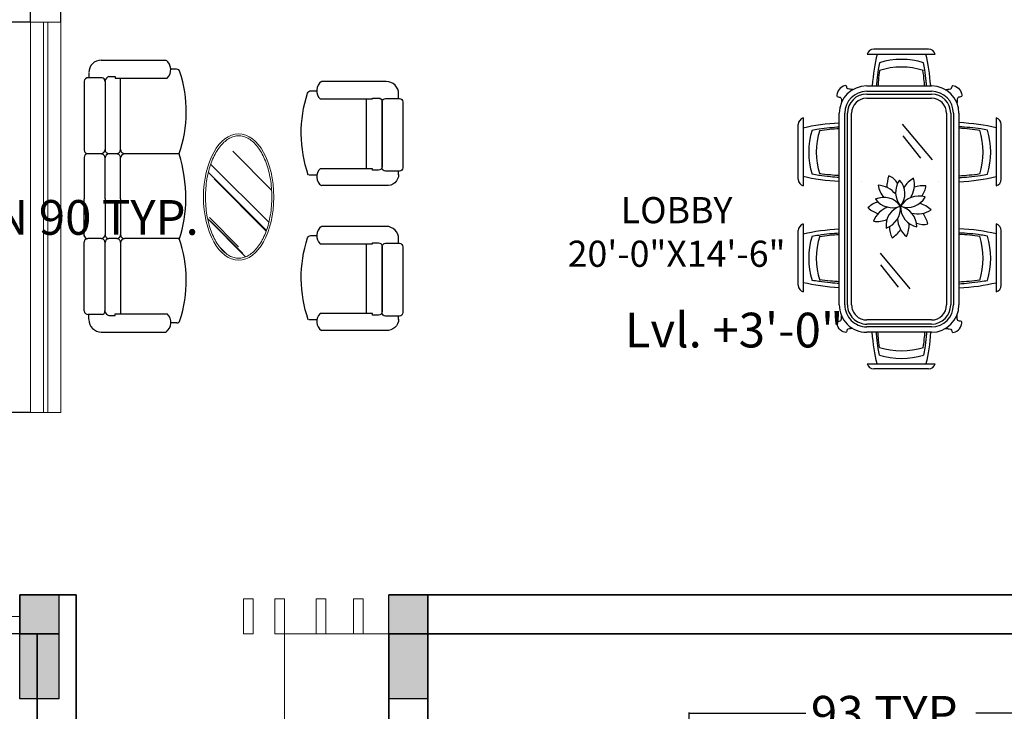
# Model space of a CAD drawing. Units: inches. Extents: x -48 to 50072, y 0 to 21068.
# Tile 52 of 75: x 212 to 439, y 660 to 819. Entities that reach past the tile are written whole.
import ezdxf

# ---------------------------------------------------------------- set-up
doc = ezdxf.new("R2010")
doc.units = ezdxf.units.IN
doc.header["$MEASUREMENT"] = 0
for name, color, linetype, lineweight in [('A-ANNO-DIMS', 2, 'Continuous', 18), ('A-ANNO-SYMB', 7, 'Continuous', 18), ('A-AREA-IDEN', 7, 'Continuous', 18), ('A-COLS', 1, 'Continuous', 35), ('A-DOOR', 4, 'Continuous', 18), ('A-FLOR-CASE', 9, 'Continuous', 18), ('A-FLOR-SCRN', 32, 'Continuous', 18), ('A-WALL', 7, 'Continuous', 35), ('FURNITURE', 44, 'Continuous', 18)]:
    doc.layers.add(name, color=color, linetype=linetype, lineweight=lineweight)
doc.layers.add('BLOCKS', color=7, linetype='Continuous')
doc.styles.get("Standard").update_dxf_attribs({"font": 'arial.ttf'})
doc.dimstyles.get("Standard").update_dxf_attribs({"dimtxt": 8, "dimasz": 0.18, "dimexe": 0.18, "dimexo": 0.0625, "dimgap": 0.09, "dimtad": 0, "dimtih": 1, "dimtoh": 1, "dimdec": 1, "dimzin": 0, "dimdsep": 46, "dimlunit": 4, "dimtxsty": 'Standard', "dimblk": 'ARCHTICK', "dimcen": 0.09, "dimadec": 0, "dimazin": 0, "dimtfac": 1, "dimtdec": 1, "dimtofl": 0, "dimtmove": 0, "dimatfit": 3, "dimldrblk": 'ARCHTICK', "dimfxl": 1, "dimtolj": 1, "dimtzin": 0, "dimarcsym": 0})

# ---------------------------------------------------------------- blocks, each defined once
blk = doc.blocks.new('bnniku')
at = {"layer": 'Defpoints'}
h = blk.add_hatch(color=256, dxfattribs=at)
h.dxf.hatch_style = 1
h.paths.add_polyline_path([(767.55, 1114.04), (758.55, 1114.04), (758.55, 1090.04), (767.55, 1090.04)])
for p, q in [((758.55, 1114.04), (767.55, 1114.04)), ((758.55, 1090.04), (758.55, 1114.04)), ((767.55, 1114.04), (767.55, 1090.04)), ((767.55, 1090.04), (758.55, 1090.04))]:
    blk.add_line(p, q, dxfattribs=at)
blk = doc.blocks.new('A$C78527CD7')
at = {"layer": 'BLOCKS'}
for p, q in [((194.3, 940.6), (831.7, 940.6)), ((862.2, 785.1), (862.2, 908.9)), ((886.4, 941), (1230.1, 941)), ((1611.9, 941), (1230.1, 941)), ((1644, 785.1), (1644, 908.9)), ((2316.1, 940.8), (1678.7, 940.8)), ((119, 897.8), (162.3, 897.8)), ((162.3, 776.5), (162.3, 904.6)), ((2348.2, 776.7), (2348.2, 904.9)), ((2391.5, 898), (2348.2, 898)), ((0, 783.4), (0, 188.4)), ((189.7, 748.7), (825.8, 748.7)), ((1230.1, 748.7), (886.4, 748.7)), ((1230.1, 748.7), (1611.9, 748.7)), ((2320.7, 749), (1684.6, 749)), ((2510.5, 783.6), (2510.5, 188.7)), ((152.6, 712.4), (152.6, 656.4)), ((152.6, 656.4), (166.9, 656.4)), ((166.9, 656.4), (166.9, 174.7)), ((862.2, 641.1), (862.2, 712.3)), ((1644, 641.1), (1644, 712.3)), ((2357.9, 656.7), (2343.6, 656.7)), ((2343.6, 656.7), (2343.6, 174.9)), ((2357.9, 712.6), (2357.9, 656.7)), ((825.8, 604.7), (166.9, 604.7)), ((862.2, 64.7), (862.2, 568.3)), ((1230.1, 604.7), (890.8, 604.7)), ((1230.1, 604.7), (1607.6, 604.7)), ((1644, 64.7), (1644, 568.3)), ((1684.6, 605), (2343.6, 605)), ((84.4, 88), (84.4, 142.7)), ((2426, 88.2), (2426, 142.9))]:
    blk.add_line(p, q, dxfattribs=at)
for centre, radius, start, end in [((197.9, 905.2), 35.6, 95.74502, 180.88345), ((829.5, 907.9), 32.8, 354.28815, 86.11137), ((894.3, 908.9), 32, 90, 180), ((1611.9, 908.9), 32, 0, 90), ((1680.9, 908.1), 32.8, 93.88863, 185.71185), ((2312.6, 905.4), 35.6, 359.11655, 84.25498), ((114.4, 783.4), 114.4, 90, 180), ((2396, 783.6), 114.4, 0, 90), ((203.8, 697.4), 53.9, 104.31345, 163.90285), ((190.2, 777.3), 27.9, 181.70275, 278.5003), ((825.8, 785.1), 36.4, 270, 360), ((825.8, 712.3), 36.4, 360, 90), ((898.6, 785.1), 36.4, 180, 270), ((898.6, 785.1), 36.4, 180, 270), ((898.6, 712.3), 36.4, 90, 180), ((1607.6, 785.1), 36.4, 270, 0), ((1607.6, 785.1), 36.4, 270, 0), ((1607.6, 712.3), 36.4, 0, 90), ((1684.6, 785.4), 36.4, 180, 270), ((1684.6, 712.6), 36.4, 90, 180), ((2320.3, 777.6), 27.9, 261.4997, 358.29725), ((2306.6, 697.7), 53.9, 16.09715, 75.68655), ((825.8, 641.1), 36.4, 270, 360), ((898.6, 641.1), 36.4, 180, 270), ((1607.6, 641.1), 36.4, 270, 0), ((1684.6, 641.4), 36.4, 180, 270), ((825.8, 568.3), 36.4, 360, 90), ((898.6, 568.3), 36.4, 90, 180), ((1607.6, 568.3), 36.4, 0, 90), ((1684.6, 568.6), 36.4, 90, 180), ((88.2, 253.3), 111.2, 217.55024, 315.04859), ((2422.3, 253.5), 111.2, 224.95141, 322.44976), ((116.5, 88), 32, 180, 252.1304), ((473.6, 1195.6), 1195.8, 252.1304, 288.99111), ((1223.2, 1157.8), 1153.7, 251.35305, 270.34112), ((1237.9, 1396), 1391.8, 269.68008, 286.96386), ((2036.9, 1195.8), 1195.8, 251.00889, 287.8696), ((2394, 88.2), 32, 287.8696, 0)]:
    blk.add_arc(centre, radius, start, end, dxfattribs=at)
blk = doc.blocks.new('A$C306A54D5')
for p, q in [((1089.2, 1060.9), (1351, 1322.4)), ((1177.4, 914.8), (1567.7, 1305)), ((1232.4, 898.4), (1621.3, 1287.3)), ((1275.1, 935.7), (1625.2, 1285.9)), ((1543.9, 893.1), (1798.6, 1147.8)), ((1558.5, 910.9), (1776.7, 1129.1)), ((1534.5, 904.5), (1730.5, 1100.5)), ((1728, 969.6), (1781.9, 1023.6))]:
    blk.add_line(p, q)
blk.add_ellipse((1396.6, 1101), major_axis=(-424.8, 0), ratio=0.556174)
blk.add_open_spline([(985.2, 1101), (985.2, 1090.7), (986.6, 1080.3), (992, 1059.7), (996.1, 1049.5), (1007.1, 1029.2), (1014, 1019.1), (1030.5, 999.6), (1040.1, 990.1), (1061.9, 971.8), (1074, 963), (1100.6, 946.5), (1115.1, 938.7), (1146, 924.4), (1162.4, 917.9), (1196.9, 906.2), (1214.9, 901), (1252.2, 892.2), (1271.5, 888.6), (1310.8, 882.8), (1330.8, 880.8), (1371.2, 878.3), (1391.6, 877.9), (1432.2, 878.7), (1452.5, 880), (1492.4, 884.1), (1512.1, 886.9), (1550.5, 894.2), (1569.2, 898.7), (1605.2, 908.9), (1622.5, 914.8), (1655.3, 927.9), (1670.8, 935), (1699.6, 950.5), (1712.9, 958.8), (1737.2, 976.3), (1748.1, 985.4), (1767.2, 1004.4), (1775.5, 1014.2), (1789.2, 1034.2), (1794.7, 1044.4), (1802.9, 1064.9), (1805.6, 1075.2), (1808.4, 1095.9), (1808.4, 1106.2), (1805.6, 1126.9), (1802.9, 1137.2), (1794.7, 1157.7), (1789.2, 1167.8), (1775.4, 1187.8), (1767.2, 1197.6), (1748, 1216.6), (1737.1, 1225.8), (1712.8, 1243.3), (1699.5, 1251.6), (1670.6, 1267), (1655.2, 1274.2), (1622.4, 1287.2), (1605.1, 1293.1), (1569.1, 1303.4), (1550.4, 1307.8), (1512, 1315.1), (1492.3, 1317.9), (1452.3, 1322), (1432.1, 1323.3), (1391.4, 1324.1), (1371.1, 1323.7), (1330.7, 1321.2), (1310.6, 1319.1), (1271.3, 1313.4), (1252.1, 1309.8), (1214.8, 1300.9), (1196.8, 1295.8), (1162.3, 1284.1), (1145.9, 1277.5), (1115, 1263.2), (1100.5, 1255.5), (1073.9, 1238.9), (1061.8, 1230.2), (1040, 1211.9), (1030.4, 1202.3), (1013.9, 1182.8), (1007.1, 1172.8), (996.1, 1152.5), (992, 1142.2), (986.6, 1121.6), (985.2, 1111.3), (985.2, 1101)], degree=3, knots=[0, 0, 0, 0, 0.146129, 0.146129, 0.292258, 0.292258, 0.438387, 0.438387, 0.584516, 0.584516, 0.730645, 0.730645, 0.876774, 0.876774, 1.022902, 1.022902, 1.169031, 1.169031, 1.31516, 1.31516, 1.461289, 1.461289, 1.607418, 1.607418, 1.753547, 1.753547, 1.899676, 1.899676, 2.045805, 2.045805, 2.191934, 2.191934, 2.338063, 2.338063, 2.484192, 2.484192, 2.630321, 2.630321, 2.77645, 2.77645, 2.922579, 2.922579, 3.068707, 3.068707, 3.214836, 3.214836, 3.360965, 3.360965, 3.507094, 3.507094, 3.653223, 3.653223, 3.799352, 3.799352, 3.945481, 3.945481, 4.09161, 4.09161, 4.237739, 4.237739, 4.383868, 4.383868, 4.529997, 4.529997, 4.676126, 4.676126, 4.822255, 4.822255, 4.968383, 4.968383, 5.114512, 5.114512, 5.260641, 5.260641, 5.40677, 5.40677, 5.552899, 5.552899, 5.699028, 5.699028, 5.845157, 5.845157, 5.991286, 5.991286, 6.137415, 6.137415, 6.283185, 6.283185, 6.283185, 6.283185])
at = {"layer": 'BLOCKS'}
for p, q in [((1246.7, 2175.3), (1222.7, 2175.3)), ((2220.4, 2175.3), (2196.4, 2175.3)), ((1206, 1958.7), (737.3, 1958.7)), ((2179.7, 1958.7), (1710.9, 1958.7)), ((1248.5, 1625.2), (1248.5, 1572)), ((2222.2, 1625.2), (2222.2, 1572))]:
    blk.add_line(p, q, dxfattribs=at)
for points in [[(757.3, 2063.6, -0.414214), (733.9, 2086.9), (733.9, 2180.2, -0.414214), (757.3, 2203.6), (1199.4, 2203.6, -0.414214), (1222.7, 2180.2), (1222.7, 2086.9, -0.414214), (1199.4, 2063.6)], [(1730.9, 2063.6, -0.414214), (1707.6, 2086.9), (1707.6, 2180.2, -0.414214), (1730.9, 2203.6), (2173, 2203.6, -0.414214), (2196.4, 2180.2), (2196.4, 2086.9, -0.414214), (2173, 2063.6)]]:
    blk.add_lwpolyline(points, format="xyb", close=True, dxfattribs=at)
for points in [[(733.9, 2175.3), (703.6, 2175.3, 0.414214), (620.2, 2091.9), (620.2, 1658.6)], [(1244.2, 2175.3, -0.433237), (1320, 2091.9), (1320, 1658.6)], [(1707.6, 2175.3), (1677.2, 2175.3, 0.414214), (1593.9, 2091.9), (1593.9, 1658.6)], [(2217.9, 2175.3, -0.433237), (2293.7, 2091.9), (2293.7, 1658.6)], [(620.2, 1656.5, 0.470418), (737.3, 1648.6), (737.3, 1999.5), (731.1, 1999.5), (731.1, 2040.2, -0.414214), (754.5, 2063.6), (1193.1, 2063.6, -0.414214), (1216.4, 2040.2), (1216.4, 1999.5), (1206, 1999.5), (1206, 1648.6, 0.482727), (1320, 1656.5)], [(1593.9, 1656.5, 0.470418), (1710.9, 1648.6), (1710.9, 1999.5), (1704.8, 1999.5), (1704.8, 2040.2, -0.414214), (1728.1, 2063.6), (2166.7, 2063.6, -0.414214), (2190.1, 2040.2), (2190.1, 1999.5), (2179.7, 1999.5), (2179.7, 1648.6, 0.482727), (2293.7, 1656.5)], [(1248.5, 1568.7, -0.162236), (697.9, 1563.3, -0.325549), (681.7, 1585.5), (681.7, 1625.3)], [(2222.2, 1568.7, -0.162236), (1671.6, 1563.3, -0.325549), (1655.4, 1585.5), (1655.4, 1625.3)]]:
    blk.add_lwpolyline(points, format="xyb", dxfattribs=at)
at = {"xscale": 0.7278252318920257, "yscale": 0.7278252318920257, "zscale": 0.7278252318920257, "rotation": 180}
blk.add_blockref('A$C78527CD7', (2303.6, 748.9), dxfattribs=at)
blk = doc.blocks.new('oihgfhye')
at = {"layer": 'BLOCKS'}
for p, q in [((631.65, 780.52), (619.03, 780.52)), ((656.1, 780.52), (643.48, 780.52)), ((617.51, 779.38), (633.16, 779.38)), ((641.97, 779.38), (657.62, 779.38)), ((616.43, 770.79), (660.62, 770.79)), ((616.43, 769.53), (660.62, 769.53)), ((616.43, 768.9), (660.62, 768.9)), ((616.43, 767.95), (660.62, 767.95)), ((602.79, 749.66), (602.79, 765.31)), ((610.12, 749.55), (610.12, 764.48)), ((611.38, 749.55), (611.38, 764.48)), ((612.01, 749.55), (612.01, 764.48)), ((612.96, 749.55), (612.96, 764.48)), ((627.19, 764.7), (618.96, 757.83)), ((632.22, 765.98), (632.26, 765.98)), ((664.09, 764.48), (664.09, 749.55)), ((665.03, 764.48), (665.03, 749.55)), ((665.67, 764.48), (665.67, 749.55)), ((666.93, 764.48), (666.93, 749.55)), ((674.21, 749.66), (674.21, 765.31)), ((601.65, 763.8), (601.65, 751.18)), ((626.8, 761.99), (621.67, 757.93)), ((675.35, 763.8), (675.35, 751.18)), ((656.91, 759.57), (648.68, 752.7)), ((656.53, 756.87), (651.4, 752.8)), ((632.22, 748.35), (632.26, 748.35)), ((660.62, 746.08), (616.43, 746.08)), ((660.62, 745.14), (616.43, 745.14)), ((660.62, 744.51), (616.43, 744.51)), ((660.62, 743.24), (616.43, 743.24)), ((617.51, 734.94), (633.16, 734.94)), ((641.97, 734.94), (657.62, 734.94)), ((631.65, 733.8), (619.03, 733.8)), ((656.1, 733.8), (643.48, 733.8))]:
    blk.add_line(p, q, dxfattribs=at)
for centre, radius, start, end in [((619.03, 778.94), 1.58, 90, 163.8086), ((631.65, 778.94), 1.58, 16.1914, 90), ((643.48, 778.94), 1.58, 90, 163.8086), ((656.1, 778.94), 1.58, 16.1914, 90), ((625.41, 761.01), 17.13, 72.7033, 107.2967), ((649.87, 761.01), 17.13, 72.7033, 107.2967), ((625.41, 759.24), 17.13, 72.7033, 107.2967), ((649.87, 759.24), 17.13, 72.7033, 107.2967), ((616.43, 764.48), 6.31, 90, 180), ((616.43, 764.48), 5.05, 90, 180), ((616.43, 764.48), 4.42, 90, 180), ((660.62, 764.48), 6.31, 0, 90), ((660.62, 764.48), 5.05, 0, 90), ((660.62, 764.48), 4.42, 0, 90), ((616.43, 764.48), 3.47, 90, 180), ((660.62, 764.48), 3.47, 0, 90), ((603.23, 763.8), 1.58, 106.1914, 180), ((643, 760.31), 5.92, 136.1301, 166.4932), ((634.19, 761.39), 5.45, 344.1324, 33.6013), ((673.77, 763.8), 1.58, 0, 73.8086), ((621.16, 757.56), 17.13, 162.7033, 197.2967), ((622.93, 757.56), 17.13, 162.7033, 197.2967), ((640.48, 762.85), 7.35, 177.2105, 198.3514), ((632.67, 758.64), 4.58, 50.5086, 84.2476), ((640.57, 761.6), 5.03, 163.7761, 237.5159), ((633.51, 758.94), 4.64, 340.0447, 61.2473), ((643.89, 756.57), 7.35, 105.2105, 126.3514), ((637.48, 762.7), 4.58, 338.5086, 12.2476), ((654.07, 757.56), 17.13, 342.7033, 17.2967), ((655.83, 757.56), 17.13, 342.7033, 17.2967), ((632.9, 755.11), 5.45, 56.1324, 105.6013), ((636.65, 763.15), 5.92, 208.1301, 238.4931), ((638.03, 761.99), 4.64, 268.0447, 349.2473), ((642.74, 756.1), 5.03, 91.7761, 165.5159), ((635.02, 753.71), 4.64, 52.0447, 133.2473), ((640.56, 762.1), 5.45, 272.1324, 321.6013), ((642.26, 753.39), 5.92, 64.1301, 94.4932), ((635.04, 752.82), 4.58, 122.5086, 156.2476), ((634.67, 761.24), 5.03, 235.7761, 309.5159), ((638.48, 751.94), 5.45, 128.1324, 177.6013), ((640.47, 753.52), 4.64, 124.0447, 205.2473), ((633.19, 755.52), 5.03, 307.7761, 21.5159), ((638.18, 752.34), 5.03, 19.7761, 93.5159), ((642.33, 758.64), 4.64, 196.0447, 277.2473), ((642.83, 759.38), 4.58, 266.5086, 300.2476), ((638.98, 751.39), 7.35, 33.2105, 54.3514), ((633.46, 761.54), 7.35, 249.2105, 270.3514), ((631.99, 757.99), 5.92, 280.1301, 310.4931), ((643.21, 756.26), 5.45, 200.1324, 249.6013), ((635.45, 751.96), 5.92, 352.1301, 22.4932), ((603.23, 751.18), 1.58, 180, 253.8086), ((641.32, 753.27), 4.58, 194.5086, 228.2476), ((632.54, 754.46), 7.35, 321.2105, 342.3514), ((673.77, 751.18), 1.58, 286.1914, 0), ((616.43, 749.55), 6.31, 180, 270), ((616.43, 749.55), 5.05, 180, 270), ((616.43, 749.55), 4.42, 180, 270), ((616.43, 749.55), 3.47, 180, 270), ((660.62, 749.55), 4.42, 270, 0), ((660.62, 749.55), 6.31, 270, 0), ((660.62, 749.55), 3.47, 270, 0), ((660.62, 749.55), 5.05, 270, 0), ((625.41, 755.08), 17.13, 252.7033, 287.2967), ((649.87, 755.08), 17.13, 252.7033, 287.2967), ((619.03, 735.38), 1.58, 196.1914, 270), ((625.41, 753.32), 17.13, 252.7033, 287.2967), ((631.65, 735.38), 1.58, 270, 343.8086), ((643.48, 735.38), 1.58, 196.1914, 270), ((649.87, 753.32), 17.13, 252.7033, 287.2967), ((656.1, 735.38), 1.58, 270, 343.8086)]:
    blk.add_arc(centre, radius, start, end, dxfattribs=at)
for centre, major_axis, start_param, end_param in [((625.41, 767.92), (0, -19.93), 4.099527, 4.56758), ((625.41, 767.92), (0, -19.93), 7.99879, 8.466844), ((649.87, 767.92), (0, -19.93), 4.099527, 4.56758), ((649.87, 767.92), (0, -19.93), 7.99879, 8.466844), ((614.25, 757.56), (19.93, 0), 8.062748, 8.466844), ((614.25, 757.56), (19.93, 0), 4.099527, 4.503623)]:
    blk.add_ellipse(centre, major_axis=major_axis, ratio=0.345133, start_param=start_param, end_param=end_param, dxfattribs=at)
at = {"layer": 'BLOCKS', "extrusion": (0, 0, -1)}
for centre, major_axis, start_param, end_param in [((662.75, 757.56), (19.93, 0), 4.923784, 5.325251), ((662.75, 757.56), (19.93, 0), 0.957934, 1.359402), ((625.41, 746.41), (0, 19.93), 4.099527, 4.553045), ((625.41, 746.41), (0, 19.93), 1.730141, 2.183659), ((649.87, 746.41), (0, 19.93), 4.099527, 4.553045), ((649.87, 746.41), (0, 19.93), 1.730141, 2.183659)]:
    blk.add_ellipse(centre, major_axis=major_axis, ratio=0.345133, start_param=start_param, end_param=end_param, dxfattribs=at)
at = {"layer": 'BLOCKS'}
for points, knots in [([(620.32, 777.36), (620.23, 776.87), (620.14, 776.35), (619.93, 775.02), (619.83, 774.18), (619.66, 772.49), (619.6, 771.65), (619.55, 770.79)], [4.2084563, 4.2084563, 4.2084563, 4.2084563, 4.2962292, 4.2962292, 4.433179, 4.433179, 4.5651263, 4.5651263, 4.5651263, 4.5651263]), ([(620.38, 775.62), (620.27, 774.87), (620.17, 774.1), (620.01, 772.49), (619.95, 771.65), (619.91, 770.79)], [4.3081151, 4.3081151, 4.3081151, 4.3081151, 4.433179, 4.433179, 4.5651263, 4.5651263, 4.5651263, 4.5651263]), ([(630.83, 770.79), (630.79, 771.58), (630.74, 772.36), (630.58, 773.98), (630.48, 774.83), (630.36, 775.65)], [8.0012444, 8.0012444, 8.0012444, 8.0012444, 8.1227425, 8.1227425, 8.2598231, 8.2598231, 8.2598231, 8.2598231]), ([(631.27, 770.79), (631.23, 771.58), (631.18, 772.36), (631.02, 774.02), (630.91, 774.91), (630.7, 776.31), (630.61, 776.84), (630.51, 777.36)], [8.0012444, 8.0012444, 8.0012444, 8.0012444, 8.1227425, 8.1227425, 8.2664644, 8.2664644, 8.3579144, 8.3579144, 8.3579144, 8.3579144]), ([(644.77, 777.36), (644.68, 776.87), (644.59, 776.35), (644.39, 775.02), (644.28, 774.18), (644.12, 772.49), (644.05, 771.65), (644.01, 770.79)], [4.2084563, 4.2084563, 4.2084563, 4.2084563, 4.2962292, 4.2962292, 4.433179, 4.433179, 4.5651263, 4.5651263, 4.5651263, 4.5651263]), ([(644.83, 775.62), (644.72, 774.87), (644.63, 774.1), (644.47, 772.49), (644.41, 771.65), (644.36, 770.79)], [4.3081151, 4.3081151, 4.3081151, 4.3081151, 4.433179, 4.433179, 4.5651263, 4.5651263, 4.5651263, 4.5651263]), ([(655.29, 770.79), (655.25, 771.58), (655.19, 772.36), (655.03, 773.98), (654.93, 774.83), (654.81, 775.65)], [8.0012444, 8.0012444, 8.0012444, 8.0012444, 8.1227425, 8.1227425, 8.2598231, 8.2598231, 8.2598231, 8.2598231]), ([(655.73, 770.79), (655.69, 771.58), (655.63, 772.36), (655.47, 774.02), (655.36, 774.91), (655.15, 776.31), (655.06, 776.84), (654.96, 777.36)], [8.0012444, 8.0012444, 8.0012444, 8.0012444, 8.1227425, 8.1227425, 8.2664644, 8.2664644, 8.3579144, 8.3579144, 8.3579144, 8.3579144]), ([(611, 767.7), (610.97, 767.98), (610.91, 768.47), (610.75, 769.2), (609.8, 769.14), (610.51, 770.75), (611.25, 771.22), (612.65, 771.66), (612.69, 770.95), (612.85, 770.37), (613.52, 770.43), (613.95, 770.38), (614.1, 770.35)], [25.854151, 25.854151, 25.854151, 25.854151, 52.771329, 71.894905, 86.117928, 121.954734, 172.04851, 202.476174, 216.691855, 230.01003, 254.635643, 269.112988, 269.112988, 269.112988, 269.112988]), ([(666.03, 767.72), (666.06, 767.99), (666.13, 768.48), (666.28, 769.2), (667.23, 769.14), (666.52, 770.75), (665.78, 771.22), (664.38, 771.66), (664.35, 770.95), (664.19, 770.37), (663.52, 770.43), (663.09, 770.38), (662.95, 770.35)], [26.596612, 26.596612, 26.596612, 26.596612, 52.771329, 71.894905, 86.117928, 121.954734, 172.04851, 202.476174, 216.691855, 230.01003, 254.635643, 268.767944, 268.767944, 268.767944, 268.767944]), ([(610.12, 763.34), (609.76, 763.32), (609.4, 763.29), (608.14, 763.17), (607.26, 763.06), (605.86, 762.85), (605.32, 762.76), (604.8, 762.66)], [8.0663515, 8.0663515, 8.0663515, 8.0663515, 8.1227425, 8.1227425, 8.2664644, 8.2664644, 8.3579144, 8.3579144, 8.3579144, 8.3579144]), ([(610.12, 762.9), (609.76, 762.88), (609.4, 762.85), (608.19, 762.73), (607.34, 762.63), (606.52, 762.51)], [8.0663515, 8.0663515, 8.0663515, 8.0663515, 8.1227425, 8.1227425, 8.2598231, 8.2598231, 8.2598231, 8.2598231]), ([(666.93, 763.34), (667.27, 763.32), (667.61, 763.29), (668.85, 763.17), (669.74, 763.06), (671.14, 762.85), (671.67, 762.76), (672.19, 762.66)], [8.0690291, 8.0690291, 8.0690291, 8.0690291, 8.1227425, 8.1227425, 8.2664644, 8.2664644, 8.3579144, 8.3579144, 8.3579144, 8.3579144]), ([(666.93, 762.9), (667.27, 762.87), (667.61, 762.84), (668.81, 762.73), (669.66, 762.63), (670.48, 762.51)], [8.0690291, 8.0690291, 8.0690291, 8.0690291, 8.1227425, 8.1227425, 8.2598231, 8.2598231, 8.2598231, 8.2598231]), ([(604.8, 752.47), (605.3, 752.38), (605.81, 752.29), (607.15, 752.08), (607.99, 751.98), (609.27, 751.85), (609.69, 751.82), (610.12, 751.78)], [4.2084563, 4.2084563, 4.2084563, 4.2084563, 4.2962292, 4.2962292, 4.433179, 4.433179, 4.5000191, 4.5000191, 4.5000191, 4.5000191]), ([(606.55, 752.53), (607.3, 752.42), (608.07, 752.32), (609.27, 752.21), (609.69, 752.17), (610.12, 752.14)], [4.3081151, 4.3081151, 4.3081151, 4.3081151, 4.433179, 4.433179, 4.5000191, 4.5000191, 4.5000191, 4.5000191]), ([(670.45, 752.53), (669.7, 752.42), (668.93, 752.32), (667.74, 752.21), (667.34, 752.17), (666.93, 752.14)], [4.3081151, 4.3081151, 4.3081151, 4.3081151, 4.433179, 4.433179, 4.4973415, 4.4973415, 4.4973415, 4.4973415]), ([(672.19, 752.47), (671.69, 752.38), (671.18, 752.29), (669.85, 752.08), (669, 751.98), (667.74, 751.85), (667.34, 751.82), (666.93, 751.79)], [4.2084563, 4.2084563, 4.2084563, 4.2084563, 4.2962292, 4.2962292, 4.433179, 4.433179, 4.4973415, 4.4973415, 4.4973415, 4.4973415]), ([(610.99, 746.35), (610.96, 746.1), (610.9, 745.63), (610.75, 744.93), (609.8, 745), (610.51, 743.39), (611.25, 742.91), (612.65, 742.48), (612.69, 743.19), (612.85, 743.76), (613.45, 743.71), (613.83, 743.75), (613.93, 743.76)], [28.55667, 28.55667, 28.55667, 28.55667, 52.771329, 71.894905, 86.117928, 121.954734, 172.04851, 202.476174, 216.691855, 230.01003, 254.635643, 263.792895, 263.792895, 263.792895, 263.792895]), ([(666.04, 746.33), (666.07, 746.09), (666.14, 745.62), (666.28, 744.93), (667.23, 745), (666.52, 743.39), (665.78, 742.91), (664.38, 742.48), (664.35, 743.19), (664.19, 743.76), (663.59, 743.71), (663.21, 743.75), (663.12, 743.76)], [29.290825, 29.290825, 29.290825, 29.290825, 52.771329, 71.894905, 86.117928, 121.954734, 172.04851, 202.476174, 216.691855, 230.01003, 254.635643, 263.419397, 263.419397, 263.419397, 263.419397]), ([(620.32, 736.96), (620.23, 737.46), (620.14, 737.97), (619.93, 739.31), (619.83, 740.15), (619.67, 741.74), (619.61, 742.49), (619.57, 743.24)], [4.2084563, 4.2084563, 4.2084563, 4.2084563, 4.2962292, 4.2962292, 4.433179, 4.433179, 4.5503345, 4.5503345, 4.5503345, 4.5503345]), ([(620.38, 738.7), (620.27, 739.45), (620.17, 740.22), (620.02, 741.74), (619.97, 742.49), (619.92, 743.24)], [4.3081151, 4.3081151, 4.3081151, 4.3081151, 4.433179, 4.433179, 4.5503345, 4.5503345, 4.5503345, 4.5503345]), ([(630.82, 743.24), (630.78, 742.56), (630.73, 741.87), (630.58, 740.34), (630.48, 739.5), (630.36, 738.68)], [8.0160361, 8.0160361, 8.0160361, 8.0160361, 8.1227425, 8.1227425, 8.2598231, 8.2598231, 8.2598231, 8.2598231]), ([(631.26, 743.24), (631.22, 742.56), (631.17, 741.87), (631.02, 740.3), (630.91, 739.41), (630.7, 738.01), (630.61, 737.48), (630.51, 736.96)], [8.0160361, 8.0160361, 8.0160361, 8.0160361, 8.1227425, 8.1227425, 8.2664644, 8.2664644, 8.3579144, 8.3579144, 8.3579144, 8.3579144]), ([(644.77, 736.96), (644.68, 737.46), (644.59, 737.97), (644.39, 739.31), (644.28, 740.15), (644.12, 741.74), (644.07, 742.49), (644.02, 743.24)], [4.2084563, 4.2084563, 4.2084563, 4.2084563, 4.2962292, 4.2962292, 4.433179, 4.433179, 4.5503345, 4.5503345, 4.5503345, 4.5503345]), ([(644.83, 738.7), (644.72, 739.45), (644.63, 740.22), (644.48, 741.74), (644.42, 742.49), (644.38, 743.24)], [4.3081151, 4.3081151, 4.3081151, 4.3081151, 4.433179, 4.433179, 4.5503345, 4.5503345, 4.5503345, 4.5503345]), ([(655.27, 743.24), (655.23, 742.56), (655.18, 741.87), (655.03, 740.34), (654.93, 739.5), (654.81, 738.68)], [8.0160361, 8.0160361, 8.0160361, 8.0160361, 8.1227425, 8.1227425, 8.2598231, 8.2598231, 8.2598231, 8.2598231]), ([(655.71, 743.24), (655.67, 742.56), (655.62, 741.87), (655.47, 740.3), (655.36, 739.41), (655.15, 738.01), (655.06, 737.48), (654.96, 736.96)], [8.0160361, 8.0160361, 8.0160361, 8.0160361, 8.1227425, 8.1227425, 8.2664644, 8.2664644, 8.3579144, 8.3579144, 8.3579144, 8.3579144])]:
    blk.add_open_spline(points, degree=3, knots=knots, dxfattribs=at)
blk = doc.blocks.new('DOOR-ENTRY-TANDEM-48')
for p, q in [((2, 43), (2, 86)), ((3, 85.99), (3, 43)), ((0, 45), (2, 45)), ((2, 41), (2, 45)), ((46, 41), (46, 45)), ((46, 45), (48, 45)), ((0, 41), (48, 41)), ((2, 43), (3, 43)), ((2, 43), (3, 43)), ((2, 43), (3, 43)), ((45, 0), (45, 43)), ((45, 43), (46, 43)), ((46, 43), (46, 7)), ((46, 7), (46, 0.01))]:
    blk.add_line(p, q)
for centre, start, end in [((2, 43), 0, 90), ((45, 43), 180, 271.3326)]:
    blk.add_arc(centre, 43, start, end)
blk = doc.blocks.new('SCREEN-JALI-90')
for p, q in [((7, 90), (0, 90)), ((0, 90), (0, 0)), ((3, 90), (3, 0)), ((4, 90), (4, 0)), ((7, 0), (7, 90)), ((7, 0), (0, 0))]:
    blk.add_line(p, q)
blk = doc.blocks.new('_ArchTick')
at = {"color": 0, "linetype": 'ByBlock', "const_width": 0.15}
blk.add_lwpolyline([(-0.5, -0.5), (0.5, 0.5)], dxfattribs=at)
blk = doc.blocks.new('*D75')
at = {"layer": 'A-ANNO-DIMS', "color": 0, "lineweight": -2, "transparency": 16777216}
for p, q in [((366.2, 638.78), (366.2, 659.65)), ((366.2, 659.47), (393.1, 659.47)), ((459.12, 659.47), (432.22, 659.47)), ((459.12, 638.78), (459.12, 659.65))]:
    blk.add_line(p, q, dxfattribs=at)
at = {"layer": 'Defpoints', "color": 0, "transparency": 16777216}
for p in [(459.12, 659.47), (366.2, 638.72), (459.12, 638.72)]:
    blk.add_point(p, dxfattribs=at)
at = {"layer": 'A-ANNO-DIMS', "color": 0, "lineweight": -2, "transparency": 16777216, "xscale": 0.18, "yscale": 0.18, "zscale": 0.18, "rotation": 180}
blk.add_blockref('_ArchTick', (366.2, 659.47), dxfattribs=at)
at = {"layer": 'A-ANNO-DIMS', "color": 0, "lineweight": -2, "transparency": 16777216, "xscale": 0.18, "yscale": 0.18, "zscale": 0.18}
blk.add_blockref('_ArchTick', (459.12, 659.47), dxfattribs=at)
at = {"layer": 'A-ANNO-DIMS', "color": 0, "transparency": 16777216, "insert": (412.66, 659.47), "char_height": 8, "attachment_point": 5}
blk.add_mtext('\\A1;93 TYP.', dxfattribs=at)
blk = doc.blocks.new('*D100')
at = {"layer": 'A-ANNO-DIMS', "color": 0, "lineweight": -2, "transparency": 16777216}
for p, q in [((214.45, 818.77), (200.84, 818.77)), ((201.02, 818.77), (201.02, 778)), ((201.02, 728.77), (201.02, 769.55)), ((214.45, 728.77), (200.84, 728.77))]:
    blk.add_line(p, q, dxfattribs=at)
at = {"layer": 'Defpoints', "color": 0, "transparency": 16777216}
for p in [(201.02, 818.77), (214.52, 818.77), (214.52, 728.77)]:
    blk.add_point(p, dxfattribs=at)
at = {"layer": 'A-ANNO-DIMS', "color": 0, "lineweight": -2, "transparency": 16777216, "xscale": 0.18, "yscale": 0.18, "zscale": 0.18}
for p, rotation in [((201.02, 818.77), 90), ((201.02, 728.77), 270)]:
    blk.add_blockref('_ArchTick', p, dxfattribs=dict(at, rotation=rotation))
at = {"layer": 'A-ANNO-DIMS', "color": 0, "transparency": 16777216, "insert": (201.02, 773.77), "char_height": 8, "attachment_point": 5}
blk.add_mtext('\\A1;JALI SCREEN 90 TYP.', dxfattribs=at)
blk = doc.blocks.new('*D101')
at = {"layer": 'A-ANNO-DIMS', "color": 0, "lineweight": -2, "transparency": 16777216}
for p, q in [((214.52, 818.84), (214.52, 832.45)), ((214.52, 832.27), (221.52, 832.27)), ((221.52, 818.84), (221.52, 832.45)), ((221.52, 832.27), (221.7, 832.27))]:
    blk.add_line(p, q, dxfattribs=at)
at = {"layer": 'Defpoints', "color": 0, "transparency": 16777216}
for p in [(221.52, 832.27), (214.52, 818.77), (221.52, 818.77)]:
    blk.add_point(p, dxfattribs=at)
at = {"layer": 'A-ANNO-DIMS', "color": 0, "lineweight": -2, "transparency": 16777216, "xscale": 0.18, "yscale": 0.18, "zscale": 0.18, "rotation": 180}
blk.add_blockref('_ArchTick', (214.52, 832.27), dxfattribs=at)
at = {"layer": 'A-ANNO-DIMS', "color": 0, "lineweight": -2, "transparency": 16777216, "xscale": 0.18, "yscale": 0.18, "zscale": 0.18}
blk.add_blockref('_ArchTick', (221.52, 832.27), dxfattribs=at)
at = {"layer": 'A-ANNO-DIMS', "color": 0, "transparency": 16777216, "insert": (238.12, 832.27), "char_height": 8, "attachment_point": 5}
blk.add_mtext('\\A1;7 TYP.', dxfattribs=at)
blk = doc.blocks.new('*D116')
at = {"layer": 'A-ANNO-DIMS', "color": 0, "lineweight": -2, "transparency": 16777216}
for p, q in [((18.02, 677.71), (18.02, 165.94)), ((216.02, 677.71), (216.02, 165.94)), ((18.02, 166.12), (108.46, 166.12)), ((216.02, 166.12), (125.58, 166.12))]:
    blk.add_line(p, q, dxfattribs=at)
at = {"layer": 'Defpoints', "color": 0, "transparency": 16777216}
for p in [(18.02, 677.77), (216.02, 677.77), (216.02, 166.12)]:
    blk.add_point(p, dxfattribs=at)
at = {"layer": 'A-ANNO-DIMS', "color": 0, "lineweight": -2, "transparency": 16777216, "xscale": 0.18, "yscale": 0.18, "zscale": 0.18, "rotation": 180}
blk.add_blockref('_ArchTick', (18.02, 166.12), dxfattribs=at)
at = {"layer": 'A-ANNO-DIMS', "color": 0, "lineweight": -2, "transparency": 16777216, "xscale": 0.18, "yscale": 0.18, "zscale": 0.18}
blk.add_blockref('_ArchTick', (216.02, 166.12), dxfattribs=at)
at = {"layer": 'A-ANNO-DIMS', "color": 0, "transparency": 16777216, "insert": (117.02, 166.12), "char_height": 8, "attachment_point": 5}
blk.add_mtext('\\A1;198', dxfattribs=at)
blk = doc.blocks.new('*D127')
at = {"layer": 'A-ANNO-DIMS', "color": 0, "lineweight": -2, "transparency": 16777216}
for p, q in [((215.95, 677.77), (-34.61, 677.77)), ((-34.43, 677.77), (-34.43, 587.45)), ((-34.43, 488.77), (-34.43, 579.1)), ((215.95, 488.77), (-34.61, 488.77))]:
    blk.add_line(p, q, dxfattribs=at)
at = {"layer": 'Defpoints', "color": 0, "transparency": 16777216}
for p in [(-34.43, 677.77), (216.02, 677.77), (216.02, 488.77)]:
    blk.add_point(p, dxfattribs=at)
at = {"layer": 'A-ANNO-DIMS', "color": 0, "lineweight": -2, "transparency": 16777216, "xscale": 0.18, "yscale": 0.18, "zscale": 0.18}
for p, rotation in [((-34.43, 677.77), 90), ((-34.43, 488.77), 270)]:
    blk.add_blockref('_ArchTick', p, dxfattribs=dict(at, rotation=rotation))
at = {"layer": 'A-ANNO-DIMS', "color": 0, "transparency": 16777216, "insert": (-34.43, 583.27), "char_height": 8, "attachment_point": 5}
blk.add_mtext('\\A1;189', dxfattribs=at)

msp = doc.modelspace()

# ---------------------------------------------------------------- linework, layer by layer
at = {"layer": 'A-FLOR-CASE'}
for p, q in [((273.017, 625.275), (273.017, 677.775)), ((273.017, 677.775), (297.017, 677.775))]:
    msp.add_line(p, q, dxfattribs=at)
at = {"layer": 'A-FLOR-SCRN'}
for points in [[(265.758, 677.775), (263.544, 677.775), (263.544, 685.88), (265.758, 685.88)], [(273.017, 677.775), (270.803, 677.775), (270.803, 685.88), (273.017, 685.88)], [(273.017, 677.775), (270.803, 677.775), (270.803, 685.88), (273.017, 685.88)], [(273.017, 677.775), (270.803, 677.775), (270.803, 685.88), (273.017, 685.88)], [(282.501, 677.775), (280.287, 677.775), (280.287, 685.88), (282.501, 685.88)], [(291.09, 677.775), (288.876, 677.775), (288.876, 685.88), (291.09, 685.88)]]:
    msp.add_lwpolyline(points, close=True, dxfattribs=at)
at = {"layer": 'A-WALL'}
for p, q in [((212.017, 677.775), (212.017, 686.775)), ((225.017, 686.775), (212.017, 686.775)), ((225.017, 625.275), (225.017, 686.775)), ((549.017, 686.775), (297.017, 686.775)), ((306.017, 497.775), (306.017, 686.775)), ((221.017, 677.775), (212.017, 677.775)), ((216.017, 488.775), (216.017, 677.775)), ((544.517, 677.775), (297.017, 677.775)), ((297.017, 625.275), (297.017, 677.775))]:
    msp.add_line(p, q, dxfattribs=at)

# ---------------------------------------------------------------- block references
at = {"layer": 'A-COLS'}
for p in [(-546.534, -427.262), (-461.534, -427.262)]:
    msp.add_blockref('bnniku', p, dxfattribs=at)
at = {"layer": 'A-DOOR'}
msp.add_blockref('DOOR-ENTRY-TANDEM-48', (164.017, 636.775), dxfattribs=at)
at = {"layer": 'A-FLOR-SCRN'}
msp.add_blockref('SCREEN-JALI-90', (214.517, 728.775), dxfattribs=at)
at = {"layer": 'FURNITURE', "rotation": 270}
msp.add_blockref('oihgfhye', (-342.459, 1414.22), dxfattribs=at)
at = {"layer": 'FURNITURE', "xscale": 0.0343036435144511, "yscale": 0.0343036435144511, "zscale": 0.0343036435144511, "rotation": 270}
msp.add_blockref('A$C306A54D5', (224.679, 826.375), dxfattribs=at)

# ---------------------------------------------------------------- texts
at = {"layer": 'A-ANNO-SYMB', "insert": (351.367, 751.801), "char_height": 8, "attachment_point": 1}
msp.add_mtext_dynamic_manual_height_columns('Lvl. +3\'-0"', width=71.79484, gutter_width=40, heights=[0], dxfattribs=at)
at = {"layer": 'A-AREA-IDEN', "insert": (304.368, 778.458), "char_height": 6.02726, "attachment_point": 1}
msp.add_mtext_dynamic_manual_height_columns('\\pxqc;LOBBY^J20\'-0"X14\'-6"', width=117.88308, gutter_width=30.136, heights=[0], dxfattribs=at)

# ---------------------------------------------------------------- dimensions: what is measured, and where the dimension line sits
at = {"layer": 'A-ANNO-DIMS'}
for base, p1, p2, picture, middle in [((221.517, 832.275), (214.517, 818.775), (221.517, 818.775), '*D101', (238.118, 832.275)), ((459.119, 659.472), (366.197, 638.717), (459.119, 638.717), '*D75', (412.658, 659.472))]:
    dim = msp.add_linear_dim(base=base, p1=p1, p2=p2, text='<> TYP.', dimstyle='Standard', override={"dimdec": 0, "dimlfac": 1, "dimrnd": 0, "dimzin": 0, "dimdsep": 46, "dimlunit": 2}, dxfattribs=at)
    dim.commit()
    dim.dimension.update_dxf_attribs({"geometry": picture, "text_midpoint": middle})
dim = msp.add_linear_dim(base=(201.017, 818.775), p1=(214.517, 728.775), p2=(214.517, 818.775), angle=90, text='JALI SCREEN <> TYP.', dimstyle='Standard', override={"dimdec": 0, "dimlfac": 1, "dimrnd": 0, "dimzin": 0, "dimdsep": 46, "dimlunit": 2}, dxfattribs=at)
dim.commit()
dim.dimension.update_dxf_attribs({"geometry": '*D100', "text_midpoint": (201.017, 773.775)})
dim = msp.add_linear_dim(base=(-34.433, 677.775), p1=(216.017, 488.775), p2=(216.017, 677.775), angle=90, dimstyle='Standard', override={"dimdec": 0, "dimlfac": 1, "dimrnd": 0, "dimzin": 0, "dimdsep": 46, "dimlunit": 2}, dxfattribs=at)
dim.commit()
dim.dimension.update_dxf_attribs({"geometry": '*D127', "text_midpoint": (-34.433, 583.275)})
dim = msp.add_linear_dim(base=(216.017, 166.125), p1=(18.017, 677.775), p2=(216.017, 677.775), dimstyle='Standard', override={"dimdec": 0, "dimlfac": 1, "dimrnd": 0, "dimzin": 0, "dimdsep": 46, "dimlunit": 2}, dxfattribs=at)
dim.commit()
dim.dimension.update_dxf_attribs({"geometry": '*D116', "text_midpoint": (117.017, 166.125)})

doc.saveas('drawing.dxf')
